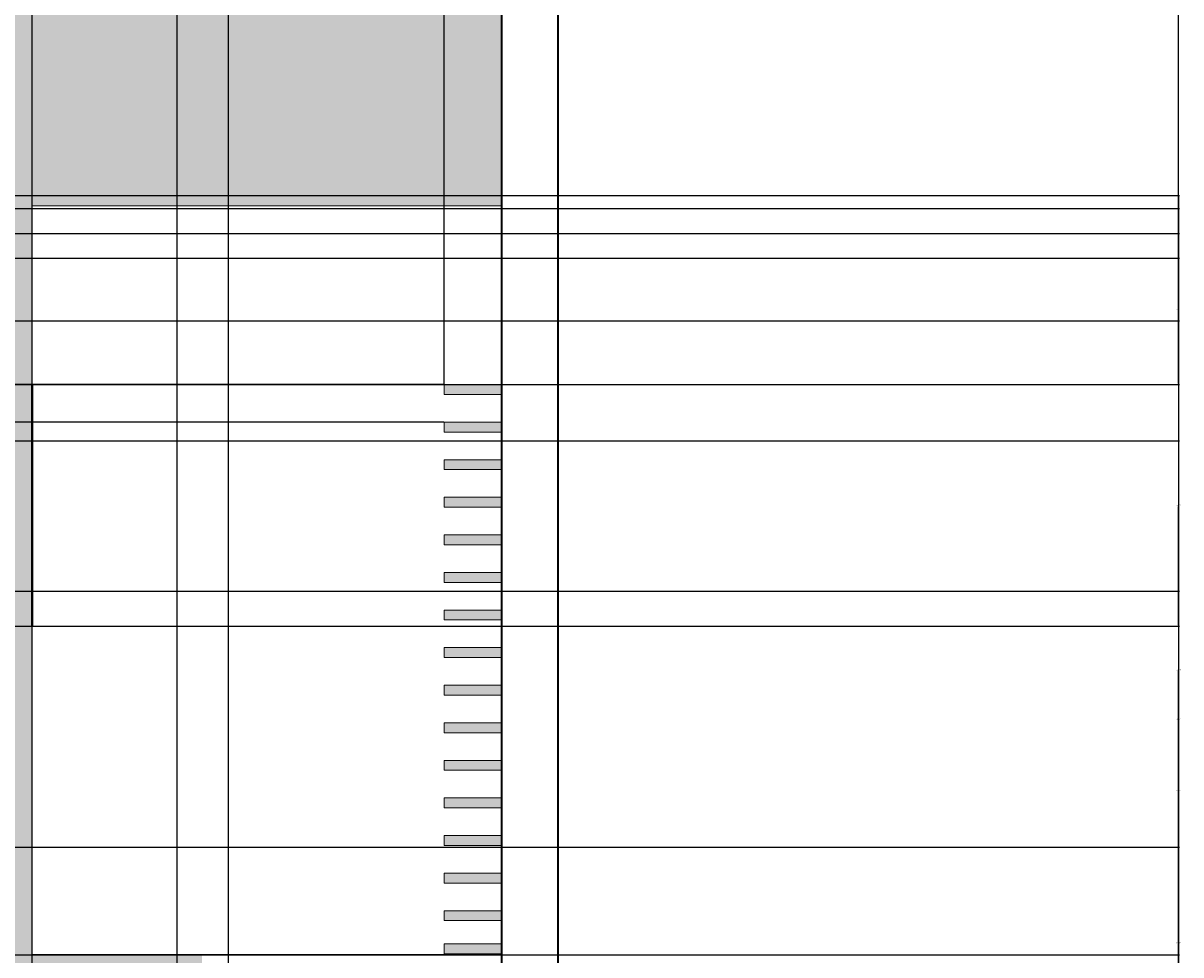
# Model space of a CAD drawing. Units: inches. Extents: x 818 to 1898, y 976 to 2364.
# Tile 93 of 96: x 1713 to 1898, y 1962 to 2111. Entities that reach past the tile are written whole.
import ezdxf

# ---------------------------------------------------------------- set-up
doc = ezdxf.new("R2010")
doc.units = ezdxf.units.IN
doc.header["$LTSCALE"] = 5
doc.header["$MEASUREMENT"] = 0
doc.linetypes.add('HIDDEN', pattern=[0.375, 0.25, -0.125])
for name, color, linetype, lineweight in [('A-ANNO-DIMS', 2, 'Continuous', 18), ('A-FLOR-SHFT', 7, 'Continuous', 25), ('A-GLAZ', 4, 'Continuous', 18), ('A-WALL', 7, 'Continuous', 40), ('A-WALL-HIDN', 7, 'HIDDEN', 18), ('C-PROP', 7, 'Continuous', 35), ('L-PAVE', 8, 'Continuous', 18)]:
    doc.layers.add(name, color=color, linetype=linetype, lineweight=lineweight)
for name, color, linetype, lineweight, true_color in [('A-GLAZ-PATT', 141, 'Continuous', 9, 0xadddf7), ('A-WALL-PATT', 251, 'Continuous', 13, 0x636466), ('L-PAVE-PATT', 9, 'Continuous', 9, 0xc7c8ca), ('L-PLNT-PATT', 114, 'Continuous', 9, 0x139b48)]:
    doc.layers.add(name, color=color, linetype=linetype, lineweight=lineweight, true_color=true_color)
doc.styles.get("Standard").update_dxf_attribs({"font": 'arial.ttf'})
doc.dimstyles.get("Standard").update_dxf_attribs({"dimtxt": 0.18, "dimasz": 0.18, "dimexe": 0.18, "dimexo": 0.0625, "dimgap": 0.09, "dimtad": 0, "dimtih": 1, "dimtoh": 1, "dimdec": 4, "dimzin": 0, "dimdsep": 46, "dimtxsty": 'Standard', "dimcen": 0.09, "dimadec": 0, "dimazin": 0, "dimtfac": 1, "dimtdec": 4, "dimtofl": 0, "dimtmove": 0, "dimatfit": 3, "dimfxl": 1, "dimtolj": 1, "dimtzin": 0, "dimarcsym": 0})

# ---------------------------------------------------------------- blocks, each defined once
blk = doc.blocks.new('*D71')
at = {"layer": 'A-ANNO-DIMS', "color": 0, "lineweight": -2, "ltscale": 5, "transparency": 16777216}
for p, q in [((1714.79, 2053.08), (1897.92, 2053.08)), ((1897.74, 2052.9), (1897.74, 1699.76)), ((1897.74, 1346.26), (1897.74, 1699.4)), ((1714.79, 1346.08), (1897.92, 1346.08))]:
    blk.add_line(p, q, dxfattribs=at)
at = {"layer": 'A-ANNO-DIMS', "color": 0, "ltscale": 5, "transparency": 16777216}
for points in [[(1897.71, 2052.9), (1897.77, 2052.9), (1897.74, 2053.08)], [(1897.71, 1346.26), (1897.77, 1346.26), (1897.74, 1346.08)]]:
    blk.add_solid(points, dxfattribs=at)
at = {"layer": 'Defpoints', "color": 0, "ltscale": 5, "transparency": 16777216}
for p in [(1714.73, 2053.08), (1897.74, 2053.08), (1714.73, 1346.08)]:
    blk.add_point(p, dxfattribs=at)
at = {"layer": 'A-ANNO-DIMS', "color": 0, "ltscale": 5, "transparency": 16777216, "insert": (1897.74, 1699.58), "char_height": 0.18, "attachment_point": 5}
blk.add_mtext('\\A1;707', dxfattribs=at)
blk = doc.blocks.new('*D72')
at = {"layer": 'A-ANNO-DIMS', "color": 0, "lineweight": -2, "ltscale": 5, "transparency": 16777216}
for p, q in [((1798.78, 2294.22), (1897.92, 2294.22)), ((1897.74, 2294.04), (1897.74, 2173.83)), ((1897.74, 2053.26), (1897.74, 2173.47)), ((1714.79, 2053.08), (1897.92, 2053.08))]:
    blk.add_line(p, q, dxfattribs=at)
at = {"layer": 'A-ANNO-DIMS', "color": 0, "ltscale": 5, "transparency": 16777216}
for points in [[(1897.71, 2294.04), (1897.77, 2294.04), (1897.74, 2294.22)], [(1897.71, 2053.26), (1897.77, 2053.26), (1897.74, 2053.08)]]:
    blk.add_solid(points, dxfattribs=at)
at = {"layer": 'Defpoints', "color": 0, "ltscale": 5, "transparency": 16777216}
for p in [(1798.72, 2294.22), (1897.74, 2294.22), (1714.73, 2053.08)]:
    blk.add_point(p, dxfattribs=at)
at = {"layer": 'A-ANNO-DIMS', "color": 0, "ltscale": 5, "transparency": 16777216, "insert": (1897.74, 2173.65), "char_height": 0.18, "attachment_point": 5}
blk.add_mtext('\\A1;241.14', dxfattribs=at)
blk = doc.blocks.new('*D85')
at = {"layer": 'A-ANNO-DIMS', "color": 0, "lineweight": -2, "ltscale": 5, "transparency": 16777216}
for p, q in [((1258.79, 2053.08), (1897.92, 2053.08)), ((1897.74, 2052.9), (1897.74, 1876.76)), ((1897.74, 1700.26), (1897.74, 1876.4)), ((1258.79, 1700.08), (1897.92, 1700.08))]:
    blk.add_line(p, q, dxfattribs=at)
at = {"layer": 'A-ANNO-DIMS', "color": 0, "ltscale": 5, "transparency": 16777216}
for points in [[(1897.71, 2052.9), (1897.77, 2052.9), (1897.74, 2053.08)], [(1897.71, 1700.26), (1897.77, 1700.26), (1897.74, 1700.08)]]:
    blk.add_solid(points, dxfattribs=at)
at = {"layer": 'Defpoints', "color": 0, "ltscale": 5, "transparency": 16777216}
for p in [(1258.73, 2053.08), (1897.74, 2053.08), (1258.73, 1700.08)]:
    blk.add_point(p, dxfattribs=at)
at = {"layer": 'A-ANNO-DIMS', "color": 0, "ltscale": 5, "transparency": 16777216, "insert": (1897.74, 1876.58), "char_height": 0.18, "attachment_point": 5}
blk.add_mtext('\\A1;353', dxfattribs=at)
blk = doc.blocks.new('*D86')
at = {"layer": 'A-ANNO-DIMS', "color": 0, "lineweight": -2, "ltscale": 5, "transparency": 16777216}
for p, q in [((1258.73, 2053.14), (1258.73, 2363.87)), ((1258.91, 2363.69), (1486.43, 2363.69)), ((1714.55, 2363.69), (1487.02, 2363.69)), ((1714.73, 2053.14), (1714.73, 2363.87))]:
    blk.add_line(p, q, dxfattribs=at)
at = {"layer": 'A-ANNO-DIMS', "color": 0, "ltscale": 5, "transparency": 16777216}
for points in [[(1258.91, 2363.72), (1258.91, 2363.66), (1258.73, 2363.69)], [(1714.55, 2363.72), (1714.55, 2363.66), (1714.73, 2363.69)]]:
    blk.add_solid(points, dxfattribs=at)
at = {"layer": 'Defpoints', "color": 0, "ltscale": 5, "transparency": 16777216}
for p in [(1714.73, 2363.69), (1258.73, 2053.08), (1714.73, 2053.08)]:
    blk.add_point(p, dxfattribs=at)
at = {"layer": 'A-ANNO-DIMS', "color": 0, "ltscale": 5, "transparency": 16777216, "insert": (1486.73, 2363.69), "char_height": 0.18, "attachment_point": 5}
blk.add_mtext('\\A1;456', dxfattribs=at)
blk = doc.blocks.new('*D104')
at = {"layer": 'A-ANNO-DIMS', "color": 0, "lineweight": -2, "ltscale": 5, "transparency": 16777216}
for p, q in [((1689.47, 1071.12), (1689.47, 2363.87)), ((1689.65, 2363.69), (1717.4, 2363.69)), ((1745.9, 2363.69), (1718.15, 2363.69)), ((1746.08, 1071.12), (1746.08, 2363.87))]:
    blk.add_line(p, q, dxfattribs=at)
at = {"layer": 'A-ANNO-DIMS', "color": 0, "ltscale": 5, "transparency": 16777216}
for points in [[(1689.65, 2363.72), (1689.65, 2363.66), (1689.47, 2363.69)], [(1745.9, 2363.72), (1745.9, 2363.66), (1746.08, 2363.69)]]:
    blk.add_solid(points, dxfattribs=at)
at = {"layer": 'Defpoints', "color": 0, "ltscale": 5, "transparency": 16777216}
for p in [(1746.08, 2363.69), (1689.47, 1071.06), (1746.08, 1071.06)]:
    blk.add_point(p, dxfattribs=at)
at = {"layer": 'A-ANNO-DIMS', "color": 0, "ltscale": 5, "transparency": 16777216, "insert": (1717.78, 2363.69), "char_height": 0.18, "attachment_point": 5}
blk.add_mtext('\\A1;56.61', dxfattribs=at)
blk = doc.blocks.new('*D141')
at = {"layer": 'A-ANNO-DIMS', "color": 0, "lineweight": -2, "ltscale": 5, "transparency": 16777216}
for p, q in [((1218.17, 2083.26), (1897.92, 2083.26)), ((1897.74, 2083.08), (1897.74, 2073.44)), ((1897.74, 2063.44), (1897.74, 2073.08)), ((1198.17, 2063.26), (1897.92, 2063.26))]:
    blk.add_line(p, q, dxfattribs=at)
at = {"layer": 'A-ANNO-DIMS', "color": 0, "ltscale": 5, "transparency": 16777216}
for points in [[(1897.71, 2083.08), (1897.77, 2083.08), (1897.74, 2083.26)], [(1897.71, 2063.44), (1897.77, 2063.44), (1897.74, 2063.26)]]:
    blk.add_solid(points, dxfattribs=at)
at = {"layer": 'Defpoints', "color": 0, "ltscale": 5, "transparency": 16777216}
for p in [(1218.11, 2083.26), (1198.11, 2063.26), (1897.74, 2063.26)]:
    blk.add_point(p, dxfattribs=at)
at = {"layer": 'A-ANNO-DIMS', "color": 0, "ltscale": 5, "transparency": 16777216, "insert": (1897.74, 2073.26), "char_height": 0.18, "attachment_point": 5}
blk.add_mtext('\\A1;20', dxfattribs=at)
blk = doc.blocks.new('*D142')
at = {"layer": 'A-ANNO-DIMS', "color": 0, "lineweight": -2, "ltscale": 5, "transparency": 16777216}
for p, q in [((1208.17, 2073.26), (1897.92, 2073.26)), ((1897.74, 2073.08), (1897.74, 2068.44)), ((1897.74, 2063.44), (1897.74, 2068.08)), ((1198.17, 2063.26), (1897.92, 2063.26))]:
    blk.add_line(p, q, dxfattribs=at)
at = {"layer": 'A-ANNO-DIMS', "color": 0, "ltscale": 5, "transparency": 16777216}
for points in [[(1897.71, 2073.08), (1897.77, 2073.08), (1897.74, 2073.26)], [(1897.71, 2063.44), (1897.77, 2063.44), (1897.74, 2063.26)]]:
    blk.add_solid(points, dxfattribs=at)
at = {"layer": 'Defpoints', "color": 0, "ltscale": 5, "transparency": 16777216}
for p in [(1208.11, 2073.26), (1897.74, 2073.26), (1198.11, 2063.26)]:
    blk.add_point(p, dxfattribs=at)
at = {"layer": 'A-ANNO-DIMS', "color": 0, "ltscale": 5, "transparency": 16777216, "insert": (1897.74, 2068.26), "char_height": 0.18, "attachment_point": 5}
blk.add_mtext('\\A1;10', dxfattribs=at)
blk = doc.blocks.new('*D186')
at = {"layer": 'A-ANNO-DIMS', "color": 0, "lineweight": -2, "ltscale": 5, "transparency": 16777216}
for p, q in [((1714.73, 1549.14), (1714.73, 2363.87)), ((1714.91, 2363.69), (1725.82, 2363.69)), ((1737.66, 2363.69), (1726.75, 2363.69)), ((1737.84, 1549.14), (1737.84, 2363.87))]:
    blk.add_line(p, q, dxfattribs=at)
at = {"layer": 'A-ANNO-DIMS', "color": 0, "ltscale": 5, "transparency": 16777216}
for points in [[(1714.91, 2363.72), (1714.91, 2363.66), (1714.73, 2363.69)], [(1737.66, 2363.72), (1737.66, 2363.66), (1737.84, 2363.69)]]:
    blk.add_solid(points, dxfattribs=at)
at = {"layer": 'Defpoints', "color": 0, "ltscale": 5, "transparency": 16777216}
for p in [(1737.84, 2363.69), (1714.73, 1549.08), (1737.84, 1549.08)]:
    blk.add_point(p, dxfattribs=at)
at = {"layer": 'A-ANNO-DIMS', "color": 0, "ltscale": 5, "transparency": 16777216, "insert": (1726.28, 2363.69), "char_height": 0.18, "attachment_point": 5}
blk.add_mtext('\\A1;23.116', dxfattribs=at)
blk = doc.blocks.new('*D204')
at = {"layer": 'A-ANNO-DIMS', "color": 0, "lineweight": -2, "ltscale": 5, "transparency": 16777216}
for p, q in [((1714.79, 2053.08), (1897.92, 2053.08)), ((1897.74, 2052.9), (1897.74, 1960.26)), ((1897.74, 1867.26), (1897.74, 1959.9)), ((1705.79, 1867.08), (1897.92, 1867.08))]:
    blk.add_line(p, q, dxfattribs=at)
at = {"layer": 'A-ANNO-DIMS', "color": 0, "ltscale": 5, "transparency": 16777216}
for points in [[(1897.71, 2052.9), (1897.77, 2052.9), (1897.74, 2053.08)], [(1897.71, 1867.26), (1897.77, 1867.26), (1897.74, 1867.08)]]:
    blk.add_solid(points, dxfattribs=at)
at = {"layer": 'Defpoints', "color": 0, "ltscale": 5, "transparency": 16777216}
for p in [(1714.73, 2053.08), (1897.74, 2053.08), (1705.73, 1867.08)]:
    blk.add_point(p, dxfattribs=at)
at = {"layer": 'A-ANNO-DIMS', "color": 0, "ltscale": 5, "transparency": 16777216, "insert": (1897.74, 1960.08), "char_height": 0.18, "attachment_point": 5}
blk.add_mtext('\\A1;186', dxfattribs=at)
blk = doc.blocks.new('*D205')
at = {"layer": 'A-ANNO-DIMS', "color": 0, "lineweight": -2, "ltscale": 5, "transparency": 16777216}
for p, q in [((1590.73, 2044.14), (1590.73, 2363.87)), ((1590.91, 2363.69), (1652.45, 2363.69)), ((1714.55, 2363.69), (1653.01, 2363.69)), ((1714.73, 2053.14), (1714.73, 2363.87))]:
    blk.add_line(p, q, dxfattribs=at)
at = {"layer": 'A-ANNO-DIMS', "color": 0, "ltscale": 5, "transparency": 16777216}
for points in [[(1590.91, 2363.72), (1590.91, 2363.66), (1590.73, 2363.69)], [(1714.55, 2363.72), (1714.55, 2363.66), (1714.73, 2363.69)]]:
    blk.add_solid(points, dxfattribs=at)
at = {"layer": 'Defpoints', "color": 0, "ltscale": 5, "transparency": 16777216}
for p in [(1714.73, 2363.69), (1714.73, 2053.08), (1590.73, 2044.08)]:
    blk.add_point(p, dxfattribs=at)
at = {"layer": 'A-ANNO-DIMS', "color": 0, "ltscale": 5, "transparency": 16777216, "insert": (1652.73, 2363.69), "char_height": 0.18, "attachment_point": 5}
blk.add_mtext('\\A1;124', dxfattribs=at)
blk = doc.blocks.new('*D208')
at = {"layer": 'A-ANNO-DIMS', "color": 0, "lineweight": -2, "ltscale": 5, "transparency": 16777216}
for p, q in [((1599.79, 2044.08), (1897.92, 2044.08)), ((1897.74, 2043.9), (1897.74, 2032.26)), ((1897.74, 2020.26), (1897.74, 2031.9)), ((1599.79, 2020.08), (1897.92, 2020.08))]:
    blk.add_line(p, q, dxfattribs=at)
at = {"layer": 'A-ANNO-DIMS', "color": 0, "ltscale": 5, "transparency": 16777216}
for points in [[(1897.71, 2043.9), (1897.77, 2043.9), (1897.74, 2044.08)], [(1897.71, 2020.26), (1897.77, 2020.26), (1897.74, 2020.08)]]:
    blk.add_solid(points, dxfattribs=at)
at = {"layer": 'Defpoints', "color": 0, "ltscale": 5, "transparency": 16777216}
for p in [(1599.73, 2044.08), (1897.74, 2044.08), (1599.73, 2020.08)]:
    blk.add_point(p, dxfattribs=at)
at = {"layer": 'A-ANNO-DIMS', "color": 0, "ltscale": 5, "transparency": 16777216, "insert": (1897.74, 2032.08), "char_height": 0.18, "attachment_point": 5}
blk.add_mtext('\\A1;24', dxfattribs=at)
blk = doc.blocks.new('*D209')
at = {"layer": 'A-ANNO-DIMS', "color": 0, "lineweight": -2, "ltscale": 5, "transparency": 16777216}
for p, q in [((1705.79, 2014.51), (1897.92, 2014.51)), ((1897.74, 2014.33), (1897.74, 1988.45)), ((1897.74, 1962.21), (1897.74, 1988.09)), ((1705.79, 1962.03), (1897.92, 1962.03))]:
    blk.add_line(p, q, dxfattribs=at)
at = {"layer": 'A-ANNO-DIMS', "color": 0, "ltscale": 5, "transparency": 16777216}
for points in [[(1897.71, 2014.33), (1897.77, 2014.33), (1897.74, 2014.51)], [(1897.71, 1962.21), (1897.77, 1962.21), (1897.74, 1962.03)]]:
    blk.add_solid(points, dxfattribs=at)
at = {"layer": 'Defpoints', "color": 0, "ltscale": 5, "transparency": 16777216}
for p in [(1705.73, 2014.51), (1897.74, 2014.51), (1705.73, 1962.03)]:
    blk.add_point(p, dxfattribs=at)
at = {"layer": 'A-ANNO-DIMS', "color": 0, "ltscale": 5, "transparency": 16777216, "insert": (1897.74, 1988.27), "char_height": 0.18, "attachment_point": 5}
blk.add_mtext('\\A1;52.48', dxfattribs=at)
blk = doc.blocks.new('*D210')
at = {"layer": 'A-ANNO-DIMS', "color": 0, "lineweight": -2, "ltscale": 5, "transparency": 16777216}
for p, q in [((1714.79, 2053.08), (1897.92, 2053.08)), ((1897.74, 2052.9), (1897.74, 2033.98)), ((1897.74, 2014.69), (1897.74, 2033.61)), ((1714.79, 2014.51), (1897.92, 2014.51))]:
    blk.add_line(p, q, dxfattribs=at)
at = {"layer": 'A-ANNO-DIMS', "color": 0, "ltscale": 5, "transparency": 16777216}
for points in [[(1897.71, 2052.9), (1897.77, 2052.9), (1897.74, 2053.08)], [(1897.71, 2014.69), (1897.77, 2014.69), (1897.74, 2014.51)]]:
    blk.add_solid(points, dxfattribs=at)
at = {"layer": 'Defpoints', "color": 0, "ltscale": 5, "transparency": 16777216}
for p in [(1714.73, 2053.08), (1897.74, 2053.08), (1714.73, 2014.51)]:
    blk.add_point(p, dxfattribs=at)
at = {"layer": 'A-ANNO-DIMS', "color": 0, "ltscale": 5, "transparency": 16777216, "insert": (1897.74, 2033.79), "char_height": 0.18, "attachment_point": 5}
blk.add_mtext('\\A1;38.57', dxfattribs=at)
blk = doc.blocks.new('*D239')
at = {"layer": 'A-ANNO-DIMS', "color": 0, "lineweight": -2, "ltscale": 5, "transparency": 16777216}
for p, q in [((1483.61, 1979.24), (1897.92, 1979.24)), ((1897.74, 1979.06), (1897.74, 1964.13)), ((1897.74, 1948.84), (1897.74, 1963.77)), ((1483.61, 1948.66), (1897.92, 1948.66))]:
    blk.add_line(p, q, dxfattribs=at)
at = {"layer": 'A-ANNO-DIMS', "color": 0, "ltscale": 5, "transparency": 16777216}
for points in [[(1897.71, 1979.06), (1897.77, 1979.06), (1897.74, 1979.24)], [(1897.71, 1948.84), (1897.77, 1948.84), (1897.74, 1948.66)]]:
    blk.add_solid(points, dxfattribs=at)
at = {"layer": 'Defpoints', "color": 0, "ltscale": 5, "transparency": 16777216}
for p in [(1483.55, 1979.24), (1897.74, 1979.24), (1483.55, 1948.66)]:
    blk.add_point(p, dxfattribs=at)
at = {"layer": 'A-ANNO-DIMS', "color": 0, "ltscale": 5, "transparency": 16777216, "insert": (1897.74, 1963.95), "char_height": 0.18, "attachment_point": 5}
blk.add_mtext('\\A1;30.584', dxfattribs=at)
blk = doc.blocks.new('*D241')
at = {"layer": 'A-ANNO-DIMS', "color": 0, "lineweight": -2, "ltscale": 5, "transparency": 16777216}
for p, q in [((1590.79, 2020.08), (1897.92, 2020.08)), ((1897.74, 2019.9), (1897.74, 1999.84)), ((1897.74, 1979.42), (1897.74, 1999.48)), ((1550.07, 1979.24), (1897.92, 1979.24))]:
    blk.add_line(p, q, dxfattribs=at)
at = {"layer": 'A-ANNO-DIMS', "color": 0, "ltscale": 5, "transparency": 16777216}
for points in [[(1897.71, 2019.9), (1897.77, 2019.9), (1897.74, 2020.08)], [(1897.71, 1979.42), (1897.77, 1979.42), (1897.74, 1979.24)]]:
    blk.add_solid(points, dxfattribs=at)
at = {"layer": 'Defpoints', "color": 0, "ltscale": 5, "transparency": 16777216}
for p in [(1590.73, 2020.08), (1897.74, 2020.08), (1550.01, 1979.24)]:
    blk.add_point(p, dxfattribs=at)
at = {"layer": 'A-ANNO-DIMS', "color": 0, "ltscale": 5, "transparency": 16777216, "insert": (1897.74, 1999.66), "char_height": 0.18, "attachment_point": 5}
blk.add_mtext('\\A1;40.83', dxfattribs=at)
blk = doc.blocks.new('*D260')
at = {"layer": 'A-ANNO-DIMS', "color": 0, "lineweight": -2, "ltscale": 5, "transparency": 16777216}
for p, q in [((1709.79, 2077.19), (1897.92, 2077.19)), ((1897.74, 2077.01), (1897.74, 2065.31)), ((1897.74, 2053.26), (1897.74, 2064.95)), ((1709.79, 2053.08), (1897.92, 2053.08))]:
    blk.add_line(p, q, dxfattribs=at)
at = {"layer": 'A-ANNO-DIMS', "color": 0, "ltscale": 5, "transparency": 16777216}
for points in [[(1897.71, 2077.01), (1897.77, 2077.01), (1897.74, 2077.19)], [(1897.71, 2053.26), (1897.77, 2053.26), (1897.74, 2053.08)]]:
    blk.add_solid(points, dxfattribs=at)
at = {"layer": 'Defpoints', "color": 0, "ltscale": 5, "transparency": 16777216}
for p in [(1709.73, 2077.19), (1897.74, 2077.19), (1709.73, 2053.08)]:
    blk.add_point(p, dxfattribs=at)
at = {"layer": 'A-ANNO-DIMS', "color": 0, "ltscale": 5, "transparency": 16777216, "insert": (1897.74, 2065.13), "char_height": 0.18, "attachment_point": 5}
blk.add_mtext('\\A1;24.11', dxfattribs=at)
blk = doc.blocks.new('*D262')
at = {"layer": 'A-ANNO-DIMS', "color": 0, "lineweight": -2, "ltscale": 5, "transparency": 16777216}
for p, q in [((1714.73, 1957.1), (1714.73, 2363.87)), ((1714.91, 2363.69), (1725.82, 2363.69)), ((1737.66, 2363.69), (1726.75, 2363.69)), ((1737.84, 1957.1), (1737.84, 2363.87))]:
    blk.add_line(p, q, dxfattribs=at)
at = {"layer": 'A-ANNO-DIMS', "color": 0, "ltscale": 5, "transparency": 16777216}
for points in [[(1714.91, 2363.72), (1714.91, 2363.66), (1714.73, 2363.69)], [(1737.66, 2363.72), (1737.66, 2363.66), (1737.84, 2363.69)]]:
    blk.add_solid(points, dxfattribs=at)
at = {"layer": 'Defpoints', "color": 0, "ltscale": 5, "transparency": 16777216}
for p in [(1737.84, 2363.69), (1714.73, 1957.03), (1737.84, 1957.03)]:
    blk.add_point(p, dxfattribs=at)
at = {"layer": 'A-ANNO-DIMS', "color": 0, "ltscale": 5, "transparency": 16777216, "insert": (1726.28, 2363.69), "char_height": 0.18, "attachment_point": 5}
blk.add_mtext('\\A1;23.116', dxfattribs=at)
blk = doc.blocks.new('*D264')
at = {"layer": 'A-ANNO-DIMS', "color": 0, "lineweight": -2, "ltscale": 5, "transparency": 16777216}
for p, q in [((1789.78, 2053.08), (1897.92, 2053.08)), ((1897.74, 2052.9), (1897.74, 2007.74)), ((1897.74, 1962.21), (1897.74, 2007.37)), ((1741.9, 1962.03), (1897.92, 1962.03))]:
    blk.add_line(p, q, dxfattribs=at)
at = {"layer": 'A-ANNO-DIMS', "color": 0, "ltscale": 5, "transparency": 16777216}
for points in [[(1897.71, 2052.9), (1897.77, 2052.9), (1897.74, 2053.08)], [(1897.71, 1962.21), (1897.77, 1962.21), (1897.74, 1962.03)]]:
    blk.add_solid(points, dxfattribs=at)
at = {"layer": 'Defpoints', "color": 0, "ltscale": 5, "transparency": 16777216}
for p in [(1789.72, 2053.08), (1897.74, 2053.08), (1741.84, 1962.03)]:
    blk.add_point(p, dxfattribs=at)
at = {"layer": 'A-ANNO-DIMS', "color": 0, "ltscale": 5, "transparency": 16777216, "insert": (1897.74, 2007.56), "char_height": 0.18, "attachment_point": 5}
blk.add_mtext('\\A1;91.04', dxfattribs=at)
blk = doc.blocks.new('*D265')
at = {"layer": 'A-ANNO-DIMS', "color": 0, "lineweight": -2, "ltscale": 5, "transparency": 16777216}
for p, q in [((1780.5, 2053.14), (1780.5, 2363.87)), ((1780.68, 2363.69), (1784.72, 2363.69)), ((1789.54, 2363.69), (1785.5, 2363.69)), ((1789.72, 2053.14), (1789.72, 2363.87))]:
    blk.add_line(p, q, dxfattribs=at)
at = {"layer": 'A-ANNO-DIMS', "color": 0, "ltscale": 5, "transparency": 16777216}
for points in [[(1780.68, 2363.72), (1780.68, 2363.66), (1780.5, 2363.69)], [(1789.54, 2363.72), (1789.54, 2363.66), (1789.72, 2363.69)]]:
    blk.add_solid(points, dxfattribs=at)
at = {"layer": 'Defpoints', "color": 0, "ltscale": 5, "transparency": 16777216}
for p in [(1789.72, 2363.69), (1780.5, 2053.08), (1789.72, 2053.08)]:
    blk.add_point(p, dxfattribs=at)
at = {"layer": 'A-ANNO-DIMS', "color": 0, "ltscale": 5, "transparency": 16777216, "insert": (1785.11, 2363.69), "char_height": 0.18, "attachment_point": 5}
blk.add_mtext('\\A1;9.215', dxfattribs=at)
blk = doc.blocks.new('*D266')
at = {"layer": 'A-ANNO-DIMS', "color": 0, "lineweight": -2, "ltscale": 5, "transparency": 16777216}
for p, q in [((1780.44, 2053.08), (818.03, 2053.08)), ((818.21, 2052.9), (818.21, 2050.26)), ((818.21, 2047.26), (818.21, 2049.9)), ((1780.44, 2047.08), (818.03, 2047.08))]:
    blk.add_line(p, q, dxfattribs=at)
at = {"layer": 'A-ANNO-DIMS', "color": 0, "ltscale": 5, "transparency": 16777216}
for points in [[(818.18, 2052.9), (818.24, 2052.9), (818.21, 2053.08)], [(818.18, 2047.26), (818.24, 2047.26), (818.21, 2047.08)]]:
    blk.add_solid(points, dxfattribs=at)
at = {"layer": 'Defpoints', "color": 0, "ltscale": 5, "transparency": 16777216}
for p in [(1780.5, 2053.08), (818.21, 2047.08), (1780.5, 2047.08)]:
    blk.add_point(p, dxfattribs=at)
at = {"layer": 'A-ANNO-DIMS', "color": 0, "ltscale": 5, "transparency": 16777216, "insert": (818.21, 2050.08), "char_height": 0.18, "attachment_point": 5}
blk.add_mtext('\\A1;6', dxfattribs=at)
blk = doc.blocks.new('*D282')
at = {"layer": 'A-ANNO-DIMS', "color": 0, "lineweight": -2, "ltscale": 5, "transparency": 16777216}
for p, q in [((1422.08, 2081.19), (1897.92, 2081.19)), ((1897.74, 2081.01), (1897.74, 1884.32)), ((1897.74, 1687.26), (1897.74, 1883.95)), ((1463.79, 1687.08), (1897.92, 1687.08))]:
    blk.add_line(p, q, dxfattribs=at)
at = {"layer": 'A-ANNO-DIMS', "color": 0, "ltscale": 5, "transparency": 16777216}
for points in [[(1897.71, 2081.01), (1897.77, 2081.01), (1897.74, 2081.19)], [(1897.71, 1687.26), (1897.77, 1687.26), (1897.74, 1687.08)]]:
    blk.add_solid(points, dxfattribs=at)
at = {"layer": 'Defpoints', "color": 0, "ltscale": 5, "transparency": 16777216}
for p in [(1422.02, 2081.19), (1897.74, 2081.19), (1463.73, 1687.08)]:
    blk.add_point(p, dxfattribs=at)
at = {"layer": 'A-ANNO-DIMS', "color": 0, "ltscale": 5, "transparency": 16777216, "insert": (1897.74, 1884.13), "char_height": 0.18, "attachment_point": 5}
blk.add_mtext('\\A1;394.1', dxfattribs=at)

msp = doc.modelspace()

# ---------------------------------------------------------------- hatches: boundary and pattern name
at = {"layer": 'A-GLAZ-PATT', "ltscale": 5}
h = msp.add_hatch(color=256, dxfattribs=at)
h.dxf.hatch_style = 1
h.paths.add_polyline_path([(1283.8183, 1504.5782), (1206.7252, 1504.5782), (1206.7252, 1501.0782), (1283.8183, 1501.0782)])
h.paths.add_polyline_path([(1283.8183, 1510.0782), (1206.7252, 1510.0782), (1206.7252, 1506.5782), (1283.8183, 1506.5782)])
h.paths.add_polyline_path([(1490.9163, 1355.0782), (1439.7252, 1355.0782), (1439.7252, 1409.0522), (1436.2252, 1409.0522), (1436.2252, 1351.5782), (1490.9163, 1351.5782)])
h.paths.add_polyline_path([(1434.2252, 1409.0522), (1430.7252, 1409.0522), (1430.7252, 1346.0782), (1435.0799, 1346.0782), (1435.0731, 1346.1152), (1435.1501, 1346.0782), (1490.9163, 1346.0782), (1490.9163, 1349.5782), (1434.2252, 1349.5782)])
h.paths.add_polyline_path([(1714.7251, 1545.0782), (1711.2252, 1545.0782), (1711.2252, 1521.0782), (1714.7251, 1521.0782)])
h.paths.add_polyline_path([(1709.2252, 1545.0782), (1705.7251, 1545.0782), (1705.7251, 1521.0782), (1709.2252, 1521.0782)])
h.paths.add_polyline_path([(1714.7251, 1687.0782), (1711.2252, 1687.0782), (1711.2252, 1649.9029), (1714.7251, 1649.9029)])
h.paths.add_polyline_path([(1709.2252, 1687.0782), (1705.7251, 1687.0782), (1705.7251, 1649.9029), (1709.2252, 1649.9029)])
h.paths.add_polyline_path([(1709.2252, 1745.5584), (1705.7251, 1745.5584), (1705.7251, 1717.3178), (1709.2252, 1717.3178)])
h.paths.add_polyline_path([(1714.7251, 1745.5584), (1711.2252, 1745.5584), (1711.2252, 1717.3178), (1714.7251, 1717.3178)])
h.paths.add_polyline_path([(1714.7251, 2014.5114), (1711.2252, 2014.5114), (1711.2252, 1962.0338), (1714.7251, 1962.0338)])
h.paths.add_polyline_path([(1709.2252, 2014.5114), (1705.7251, 2014.5114), (1705.7251, 1962.0338), (1709.2252, 1962.0338)])
h.paths.add_polyline_path([(1538.5155, 2047.5782), (1485.1216, 2047.5782), (1485.1216, 2044.0782), (1538.5155, 2044.0782)])
h.paths.add_polyline_path([(1538.5155, 2053.0782), (1485.1216, 2053.0782), (1485.1216, 2049.5782), (1538.5155, 2049.5782)])
h.paths.add_polyline_path([(1388.0315, 2047.5782), (1330.305, 2047.5782), (1330.305, 2044.0782), (1388.0315, 2044.0782)])
h.paths.add_polyline_path([(1388.0315, 2053.0782), (1330.305, 2053.0782), (1330.305, 2049.5782), (1388.0315, 2049.5782)])
h.paths.add_polyline_path([(1262.2252, 2019.2871), (1258.7251, 2019.2871), (1258.7251, 1928.9218), (1262.2252, 1928.9218)])
h.paths.add_polyline_path([(1267.7252, 2019.2871), (1264.2252, 2019.2871), (1264.2252, 1928.9218), (1267.7252, 1928.9218)])
h.paths.add_polyline_path([(1262.2252, 1862.9652), (1258.7251, 1862.9652), (1258.7251, 1814.9652), (1262.2252, 1814.9652)])
h.paths.add_polyline_path([(1267.7252, 1862.9652), (1264.2252, 1862.9652), (1264.2252, 1814.9652), (1267.7252, 1814.9652)])
h.paths.add_polyline_path([(1262.2252, 1755.3321), (1258.7251, 1755.3321), (1258.7251, 1707.3321), (1262.2252, 1707.3321)])
h.paths.add_polyline_path([(1267.7252, 1755.3321), (1264.2252, 1755.3321), (1264.2252, 1707.3321), (1267.7252, 1707.3321)])
h.paths.add_polyline_path([(1251.9333, 1692.5782), (1206.7252, 1692.5782), (1206.7252, 1687.0782), (1251.9333, 1687.0782)])
h.paths.add_polyline_path([(1251.9333, 1700.0782), (1206.7252, 1700.0782), (1206.7252, 1694.5782), (1251.9333, 1694.5782)])
at = {"layer": 'A-WALL-PATT', "ltscale": 5}
h = msp.add_hatch(color=256, dxfattribs=at)
h.dxf.hatch_style = 1
h.paths.add_polyline_path([(1267.7252, 1928.9218), (1258.7251, 1928.9218), (1258.7251, 1913.6401), (1250.3029, 1913.6401), (1250.3029, 1878.3919), (1258.7251, 1878.3919), (1258.7251, 1862.9652), (1267.7252, 1862.9652)])
h.paths.add_polyline_path([(1267.7252, 1814.9652), (1258.7251, 1814.9652), (1258.7251, 1755.3321), (1267.7252, 1755.3321)])
h.paths.add_polyline_path([(1463.7251, 1696.0782), (1267.7252, 1696.0782), (1267.7252, 1707.3321), (1258.7251, 1707.3321), (1258.7251, 1700.0782), (1251.9333, 1700.0782), (1251.9333, 1687.0782), (1463.7251, 1687.0782)])
h.paths.add_polyline_path([(1714.7251, 1717.3178), (1705.7251, 1717.3178), (1705.7251, 1696.0782), (1599.7251, 1696.0782), (1599.7251, 1790.0782), (1705.7251, 1790.0782), (1705.7251, 1785.6125), (1714.7251, 1785.6125), (1714.7251, 1827.2125), (1705.7251, 1827.2125), (1705.7251, 1802.0782), (1599.7251, 1802.0782), (1599.7251, 1867.0782), (1705.7251, 1867.0782), (1705.7251, 1857.2125), (1714.7251, 1857.2125), (1714.7251, 1930.0316), (1741.8409, 1930.0316), (1741.8409, 1935.0316), (1714.7251, 1935.0316), (1714.7251, 1957.0338), (1741.8409, 1957.0338), (1741.8409, 1962.0338), (1714.7251, 1962.0338), (1705.7251, 1962.0338), (1705.7251, 1948.0782), (1599.7251, 1948.0782), (1599.7251, 1981.0782), (1590.7251, 1981.0782), (1590.7251, 1941.0782), (1620.7252, 1941.0782), (1705.7251, 1941.0782), (1705.7251, 1876.0782), (1599.7251, 1876.0782), (1599.7251, 1911.0782), (1590.7251, 1911.0782), (1590.7251, 1876.0782), (1429.2252, 1876.0782), (1429.2252, 1867.0782), (1511.7252, 1867.0782), (1528.593, 1867.0782), (1595.7252, 1867.0782), (1595.7252, 1773.0782), (1520.7252, 1773.0782), (1520.7252, 1837.5823), (1532.593, 1837.5823), (1532.593, 1867.0782), (1528.593, 1867.0782), (1528.593, 1841.5823), (1511.7252, 1841.5823), (1511.7252, 1744.9714), (1520.7252, 1744.9714), (1520.7252, 1761.0782), (1595.7252, 1761.0782), (1595.7252, 1696.0782), (1520.7252, 1696.0782), (1520.7252, 1716.0454), (1511.7252, 1716.0454), (1511.7252, 1696.0782), (1511.7252, 1687.0782), (1714.7251, 1687.0782)])
h.paths.add_polyline_path([(1714.7251, 2053.0782), (1714.7251, 2081.1881), (1709.7251, 2081.1881), (1709.7251, 2053.0782), (1681.6446, 2053.0782), (1681.6446, 2081.1881), (1676.6446, 2081.1881), (1676.6446, 2053.0782), (1538.5155, 2053.0782), (1538.5155, 2044.0782), (1590.7251, 2044.0782), (1590.7251, 2011.0782), (1599.7251, 2011.0782), (1599.7251, 2044.0782), (1705.7251, 2044.0782), (1705.7251, 2014.5114), (1714.7251, 2014.5114)])
h.paths.add_polyline_path([(1485.1216, 2053.0782), (1422.02, 2053.0782), (1422.02, 2081.1881), (1413.02, 2081.1881), (1413.02, 2053.0782), (1399.6356, 2053.0782), (1399.6356, 2081.1881), (1390.6356, 2081.1881), (1390.6356, 2053.0782), (1388.0315, 2053.0782), (1388.0315, 2044.0782), (1416.2743, 2044.0782), (1485.1216, 2044.0782)])
h.paths.add_polyline_path([(1330.305, 2053.0782), (1258.7251, 2053.0782), (1258.7251, 2019.2871), (1267.7252, 2019.2871), (1267.7252, 2044.0782), (1330.305, 2044.0782)])
h.paths.add_polyline_path([(1258.7251, 2053.0782), (1214.6577, 2053.0782), (1214.6577, 2044.0782), (1258.7251, 2044.0782)])
h.paths.add_polyline_path([(1214.6577, 2053.0782), (1180.349, 2053.0782), (1180.349, 2044.0782), (1214.6577, 2044.0782)])
h.paths.add_polyline_path([(1714.7251, 1639.5782), (1741.8409, 1639.5782), (1741.8409, 1643.5782), (1714.7251, 1643.5782), (1714.7251, 1649.9029), (1705.7251, 1649.9029), (1705.7251, 1600.0782), (1477.7252, 1600.0782), (1477.7252, 1591.0782), (1520.7252, 1591.0782), (1616.7252, 1591.0782), (1616.7252, 1416.6857), (1622.7252, 1416.6857), (1622.7252, 1463.0782), (1624.7252, 1463.0782), (1624.7252, 1467.0782), (1622.7252, 1467.0782), (1622.7252, 1591.0782), (1705.7251, 1591.0782), (1705.7251, 1545.0782), (1714.7251, 1545.0782), (1741.8409, 1545.0782), (1741.8409, 1549.0782), (1714.7251, 1549.0782), (1714.7251, 1593.9175), (1737.8409, 1593.9175), (1737.8409, 1597.9175), (1714.7251, 1597.9175)])
h.paths.add_polyline_path([(1674.9024, 2060.7419), (1714.7045, 2060.7419), (1714.7045, 2073.1061), (1674.9024, 2073.1061)], flags=25)
h.paths.add_polyline_path([(1394.5468, 2061.6618), (1422.2344, 2061.6618), (1422.2344, 2074.0261), (1394.5468, 2074.0261)], flags=24)
at = {"layer": 'L-PAVE-PATT', "ltscale": 5}
h = msp.add_hatch(color=256, dxfattribs=at)
h.dxf.hatch_style = 1
h.paths.add_polyline_path([(1789.7173, 2053.0782), (1780.5019, 2053.0782), (1780.5019, 2051.4963), (1789.7173, 2051.4963)])
h.paths.add_polyline_path([(1789.7173, 2047.0782), (1780.5019, 2047.0782), (1780.5019, 2045.4963), (1789.7173, 2045.4963)])
h.paths.add_polyline_path([(1789.7173, 2041.0782), (1780.5019, 2041.0782), (1780.5019, 2039.4963), (1789.7173, 2039.4963)])
h.paths.add_polyline_path([(1789.7173, 2035.0782), (1780.5019, 2035.0782), (1780.5019, 2033.4963), (1789.7173, 2033.4963)])
h.paths.add_polyline_path([(1789.7173, 2029.0782), (1780.5019, 2029.0782), (1780.5019, 2027.4963), (1789.7173, 2027.4963)])
h.paths.add_polyline_path([(1789.7173, 2023.0782), (1780.5019, 2023.0782), (1780.5019, 2021.4963), (1789.7173, 2021.4963)])
h.paths.add_polyline_path([(1789.7173, 1963.7655), (1780.5019, 1963.7655), (1780.5019, 1962.1835), (1789.7173, 1962.1835)])
h.paths.add_polyline_path([(1789.7173, 1969.0782), (1780.5019, 1969.0782), (1780.5019, 1967.4963), (1789.7173, 1967.4963)])
h.paths.add_polyline_path([(1789.7173, 1975.0782), (1780.5019, 1975.0782), (1780.5019, 1973.4963), (1789.7173, 1973.4963)])
h.paths.add_polyline_path([(1789.7173, 1981.0782), (1780.5019, 1981.0782), (1780.5019, 1979.4963), (1789.7173, 1979.4963)])
h.paths.add_polyline_path([(1789.7173, 1987.0782), (1780.5019, 1987.0782), (1780.5019, 1985.4963), (1789.7173, 1985.4963)])
h.paths.add_polyline_path([(1789.7173, 1993.0782), (1780.5019, 1993.0782), (1780.5019, 1991.4963), (1789.7173, 1991.4963)])
h.paths.add_polyline_path([(1789.7173, 1999.0782), (1780.5019, 1999.0782), (1780.5019, 1997.4963), (1789.7173, 1997.4963)])
h.paths.add_polyline_path([(1789.7173, 2005.0782), (1780.5019, 2005.0782), (1780.5019, 2003.4963), (1789.7173, 2003.4963)])
h.paths.add_polyline_path([(1789.7173, 2011.0782), (1780.5019, 2011.0782), (1780.5019, 2009.4963), (1789.7173, 2009.4963)])
h.paths.add_polyline_path([(1789.7173, 2017.0782), (1780.5019, 2017.0782), (1780.5019, 2015.4963), (1789.7173, 2015.4963)])
at = {"layer": 'L-PLNT-PATT', "ltscale": 5}
h = msp.add_hatch(color=256, dxfattribs=at)
h.dxf.hatch_style = 1
h.paths.add_polyline_path([(1789.7173, 2205.9709), (1083.7252, 2205.9709), (1083.7252, 2083.2623), (1218.1114, 2083.2623), (1218.1114, 2053.0782), (1390.6356, 2053.0782), (1390.6356, 2081.1881), (1399.6356, 2081.1881), (1413.02, 2081.1881), (1422.02, 2081.1881), (1422.02, 2053.0782), (1676.6446, 2053.0782), (1676.6446, 2081.1881), (1714.7251, 2081.1881), (1714.7251, 2081.6235), (1789.7173, 2081.6235)])
h.paths.add_polyline_path([(1388.6037, 2145.2461), (1388.6037, 2122.3767), (1373.4756, 2122.3767), (1373.4756, 2145.2461)], flags=16)
h.paths.add_polyline_path([(1408.6922, 2145.2461), (1423.8203, 2145.2461), (1423.8203, 2122.3767), (1408.6922, 2122.3767)], flags=16)
h.paths.add_polyline_path([(1353.3871, 2155.7839), (1353.3871, 2122.3767), (1338.259, 2122.3767), (1338.259, 2155.7839)], flags=16)
h.paths.add_polyline_path([(1443.9089, 2158.4222), (1459.037, 2158.4222), (1459.037, 2122.3767), (1443.9089, 2122.3767)], flags=16)
h.paths.add_polyline_path([(1318.1705, 2145.2461), (1318.1705, 2122.3767), (1303.0424, 2122.3767), (1303.0424, 2145.2461)], flags=16)
h.paths.add_polyline_path([(1479.1255, 2145.2461), (1494.2536, 2145.2461), (1494.2536, 2122.3767), (1479.1255, 2122.3767)], flags=16)
h.paths.add_polyline_path([(1282.9539, 2145.2461), (1282.9539, 2122.3767), (1267.8258, 2122.3767), (1267.8258, 2145.2461)], flags=16)
h.paths.add_polyline_path([(1514.3421, 2145.2461), (1529.4702, 2145.2461), (1529.4702, 2122.3767), (1514.3421, 2122.3767)], flags=16)
h.paths.add_polyline_path([(1247.7373, 2159.4296), (1247.7373, 2122.3767), (1232.6091, 2122.3767), (1232.6091, 2159.4296)], flags=16)
h.paths.add_polyline_path([(1549.5587, 2156.9246), (1564.6868, 2156.9246), (1564.6868, 2122.3767), (1549.5587, 2122.3767)], flags=16)
h.paths.add_polyline_path([(1212.5206, 2145.2461), (1212.5206, 2122.3767), (1197.3925, 2122.3767), (1197.3925, 2145.2461)], flags=16)
h.paths.add_polyline_path([(1584.7753, 2145.2461), (1599.9034, 2145.2461), (1599.9034, 2122.3767), (1584.7753, 2122.3767)], flags=16)
h.paths.add_polyline_path([(1185.1073, 2104.7786), (1190.6407, 2104.7786), (1185.1073, 2098.2505), (1179.5738, 2104.7786)], flags=16)
h.paths.add_polyline_path([(1619.9919, 2145.2461), (1635.1201, 2145.2461), (1635.1201, 2122.3767), (1619.9919, 2122.3767)], flags=16)
h.paths.add_polyline_path([(1655.2086, 2156.1761), (1670.3367, 2156.1761), (1670.3367, 2122.3767), (1655.2086, 2122.3767)], flags=16)
h.paths.add_polyline_path([(1686.5992, 2145.2461), (1701.7273, 2145.2461), (1701.7273, 2122.3767), (1686.5992, 2122.3767)], flags=16)
h.paths.add_polyline_path([(1715.7616, 2145.2461), (1730.8897, 2145.2461), (1730.8897, 2122.3767), (1715.7616, 2122.3767)], flags=16)
h.paths.add_polyline_path([(1753.1652, 2145.2461), (1776.3312, 2145.2461), (1776.3312, 2115.6891), (1753.1652, 2115.6891)], flags=16)
h.paths.add_polyline_path([(1191.4331, 2146.5159), (1176.7891, 2146.5159), (1176.7891, 2134.1516), (1191.4331, 2134.1516)], flags=24)

# ---------------------------------------------------------------- linework, layer by layer
at = {"layer": 'A-FLOR-SHFT'}
for p in [(1676.6446, 2081.1881), (1714.7251, 2053.0782)]:
    msp.add_line(p, (1714.7251, 2081.1881), dxfattribs=at)
at = {"layer": 'A-GLAZ'}
msp.add_line((1705.7251, 2014.5114), (1714.7251, 2014.5114), dxfattribs=at)
at = {"layer": 'A-WALL'}
msp.add_line((1714.7251, 2053.0782), (1714.7251, 2014.5114), dxfattribs=at)
at = {"layer": 'A-WALL-HIDN', "ltscale": 5}
msp.add_line((1714.7355, 2013.5614), (1714.7355, 1962.0338), dxfattribs=at)
at = {"layer": 'C-PROP', "ltscale": 5}
for p, q in [((1798.7173, 1202.9642), (1798.7173, 2294.2171)), ((1789.7173, 1211.9642), (1789.7173, 2285.2171))]:
    msp.add_line(p, q, dxfattribs=at)
at = {"layer": 'L-PAVE', "ltscale": 5}
for points in [[(1714.7251, 2053.0782), (1789.7173, 2053.0782), (1789.7173, 2081.6235), (1714.7251, 2081.6235)], [(1714.7251, 2053.0782), (1789.7173, 2053.0782), (1789.7173, 1962.0641), (1714.7251, 1962.0641)], [(1780.5019, 2053.0782), (1789.7173, 2053.0782), (1789.7173, 2051.4963), (1780.5019, 2051.4963)], [(1780.5019, 2047.0782), (1789.7173, 2047.0782), (1789.7173, 2045.4963), (1780.5019, 2045.4963)], [(1780.5019, 2041.0782), (1789.7173, 2041.0782), (1789.7173, 2039.4963), (1780.5019, 2039.4963)], [(1780.5019, 2035.0782), (1789.7173, 2035.0782), (1789.7173, 2033.4963), (1780.5019, 2033.4963)], [(1780.5019, 2029.0782), (1789.7173, 2029.0782), (1789.7173, 2027.4963), (1780.5019, 2027.4963)], [(1780.5019, 2023.0782), (1789.7173, 2023.0782), (1789.7173, 2021.4963), (1780.5019, 2021.4963)], [(1780.5019, 2017.0782), (1789.7173, 2017.0782), (1789.7173, 2015.4963), (1780.5019, 2015.4963)], [(1780.5019, 2011.0782), (1789.7173, 2011.0782), (1789.7173, 2009.4963), (1780.5019, 2009.4963)], [(1780.5019, 2005.0782), (1789.7173, 2005.0782), (1789.7173, 2003.4963), (1780.5019, 2003.4963)], [(1780.5019, 1999.0782), (1789.7173, 1999.0782), (1789.7173, 1997.4963), (1780.5019, 1997.4963)], [(1780.5019, 1993.0782), (1789.7173, 1993.0782), (1789.7173, 1991.4963), (1780.5019, 1991.4963)], [(1780.5019, 1987.0782), (1789.7173, 1987.0782), (1789.7173, 1985.4963), (1780.5019, 1985.4963)], [(1780.5019, 1981.0782), (1789.7173, 1981.0782), (1789.7173, 1979.4963), (1780.5019, 1979.4963)], [(1780.5019, 1975.0782), (1789.7173, 1975.0782), (1789.7173, 1973.4963), (1780.5019, 1973.4963)], [(1780.5019, 1969.0782), (1789.7173, 1969.0782), (1789.7173, 1967.4963), (1780.5019, 1967.4963)], [(1780.5019, 1963.7655), (1789.7173, 1963.7655), (1789.7173, 1962.1835), (1780.5019, 1962.1835)]]:
    msp.add_lwpolyline(points, close=True, dxfattribs=at)

# ---------------------------------------------------------------- dimensions: what is measured, and where the dimension line sits
at = {"layer": 'A-ANNO-DIMS', "ltscale": 5}
for base, p1, p2, override, picture, middle in [((1714.7251, 2363.6929), (1258.7251, 2053.0782), (1714.7251, 2053.0782), {"dimdec": 0, "dimlfac": 1, "dimrnd": 0, "dimzin": 0, "dimdsep": 46, "dimlunit": 2}, '*D86', (1486.7251, 2363.6929)), ((1714.7251, 2363.6929), (1590.7251, 2044.0782), (1714.7251, 2053.0782), {"dimdec": 0, "dimlfac": 1, "dimrnd": 0, "dimzin": 0, "dimdsep": 46, "dimlunit": 2}, '*D205', (1652.7251, 2363.6929)), ((1746.0831, 2363.6929), (1689.4714, 1071.0552), (1746.0831, 1071.0552), {"dimdec": 2, "dimlfac": 1, "dimrnd": 0, "dimzin": 0, "dimdsep": 46, "dimlunit": 2}, '*D104', (1717.7772, 2363.6929)), ((1737.8409, 2363.6929), (1714.7251, 1549.0782), (1737.8409, 1549.0782), {"dimdec": 3, "dimlfac": 1, "dimrnd": 0, "dimzin": 0, "dimdsep": 46, "dimlunit": 2}, '*D186', (1726.283, 2363.6929)), ((1737.8409, 2363.6929), (1714.7251, 1957.0338), (1737.8409, 1957.0338), {"dimdec": 3, "dimlfac": 1, "dimrnd": 0, "dimzin": 0, "dimdsep": 46, "dimlunit": 2}, '*D262', (1726.283, 2363.6929)), ((1789.7173, 2363.6929), (1780.5019, 2053.0782), (1789.7173, 2053.0782), {"dimdec": 3, "dimlfac": 1, "dimrnd": 0, "dimzin": 0, "dimdsep": 46, "dimlunit": 2}, '*D265', (1785.1096, 2363.6929))]:
    dim = msp.add_linear_dim(base=base, p1=p1, p2=p2, dimstyle='Standard', override=override, dxfattribs=at)
    dim.commit()
    dim.dimension.update_dxf_attribs({"geometry": picture, "text_midpoint": middle})
for base, p1, p2, override, picture, middle in [((1897.736, 2294.2171), (1714.7251, 2053.0782), (1798.7173, 2294.2171), {"dimdec": 2, "dimlfac": 1, "dimrnd": 0, "dimzin": 0, "dimdsep": 46, "dimlunit": 2}, '*D72', (1897.736, 2173.6477)), ((1897.736, 2063.2623), (1218.1114, 2083.2623), (1198.1114, 2063.2623), {"dimdec": 0, "dimlfac": 1, "dimrnd": 0, "dimzin": 0, "dimdsep": 46, "dimlunit": 2}, '*D141', (1897.736, 2073.2623)), ((1897.736, 2081.1881), (1463.7251, 1687.0782), (1422.02, 2081.1881), {"dimdec": 1, "dimlfac": 1, "dimrnd": 0, "dimzin": 0, "dimdsep": 46, "dimlunit": 2}, '*D282', (1897.736, 1884.1332)), ((1897.736, 2077.1881), (1709.7251, 2053.0782), (1709.7251, 2077.1881), {"dimdec": 2, "dimlfac": 1, "dimrnd": 0, "dimzin": 0, "dimdsep": 46, "dimlunit": 2}, '*D260', (1897.736, 2065.1332)), ((1897.736, 2073.2623), (1198.1114, 2063.2623), (1208.1114, 2073.2623), {"dimdec": 0, "dimlfac": 1, "dimrnd": 0, "dimzin": 0, "dimdsep": 46, "dimlunit": 2}, '*D142', (1897.736, 2068.2623)), ((818.2059, 2047.0782), (1780.5019, 2053.0782), (1780.5019, 2047.0782), {"dimdec": 0, "dimlfac": 1, "dimrnd": 0, "dimzin": 0, "dimdsep": 46, "dimlunit": 2}, '*D266', (818.2059, 2050.0782)), ((1897.736, 2053.0782), (1258.7251, 1700.0782), (1258.7251, 2053.0782), {"dimdec": 0, "dimlfac": 1, "dimrnd": 0, "dimzin": 0, "dimdsep": 46, "dimlunit": 2}, '*D85', (1897.736, 1876.5782)), ((1897.736, 2053.0782), (1705.7251, 1867.0782), (1714.7251, 2053.0782), {"dimdec": 0, "dimlfac": 1, "dimrnd": 0, "dimzin": 0, "dimdsep": 46, "dimlunit": 2}, '*D204', (1897.736, 1960.0782)), ((1897.736, 2053.0782), (1714.7251, 1346.0782), (1714.7251, 2053.0782), {"dimdec": 0, "dimlfac": 1, "dimrnd": 0, "dimzin": 0, "dimdsep": 46, "dimlunit": 2}, '*D71', (1897.736, 1699.5782)), ((1897.736, 2053.0782), (1714.7251, 2014.5114), (1714.7251, 2053.0782), {"dimdec": 2, "dimlfac": 1, "dimrnd": 0, "dimzin": 0, "dimdsep": 46, "dimlunit": 2}, '*D210', (1897.736, 2033.7948)), ((1897.736, 2053.0782), (1741.8409, 1962.0338), (1789.7173, 2053.0782), {"dimdec": 2, "dimlfac": 1, "dimrnd": 0, "dimzin": 0, "dimdsep": 46, "dimlunit": 2}, '*D264', (1897.736, 2007.556)), ((1897.736, 2044.0782), (1599.7251, 2020.0782), (1599.7251, 2044.0782), {"dimdec": 0, "dimlfac": 1, "dimrnd": 0, "dimzin": 0, "dimdsep": 46, "dimlunit": 2}, '*D208', (1897.736, 2032.0782)), ((1897.736, 2020.0782), (1550.0109, 1979.2444), (1590.7251, 2020.0782), {"dimdec": 2, "dimlfac": 1, "dimrnd": 0, "dimzin": 0, "dimdsep": 46, "dimlunit": 2}, '*D241', (1897.736, 1999.6613)), ((1897.736, 2014.5114), (1705.7251, 1962.0338), (1705.7251, 2014.5114), {"dimdec": 2, "dimlfac": 1, "dimrnd": 0, "dimzin": 0, "dimdsep": 46, "dimlunit": 2}, '*D209', (1897.736, 1988.2726)), ((1897.736, 1979.2444), (1483.5451, 1948.6602), (1483.5451, 1979.2444), {"dimdec": 3, "dimlfac": 1, "dimrnd": 0, "dimzin": 0, "dimdsep": 46, "dimlunit": 2}, '*D239', (1897.736, 1963.9523))]:
    dim = msp.add_linear_dim(base=base, p1=p1, p2=p2, angle=90, dimstyle='Standard', override=override, dxfattribs=at)
    dim.commit()
    dim.dimension.update_dxf_attribs({"geometry": picture, "text_midpoint": middle})

doc.saveas('drawing.dxf')
